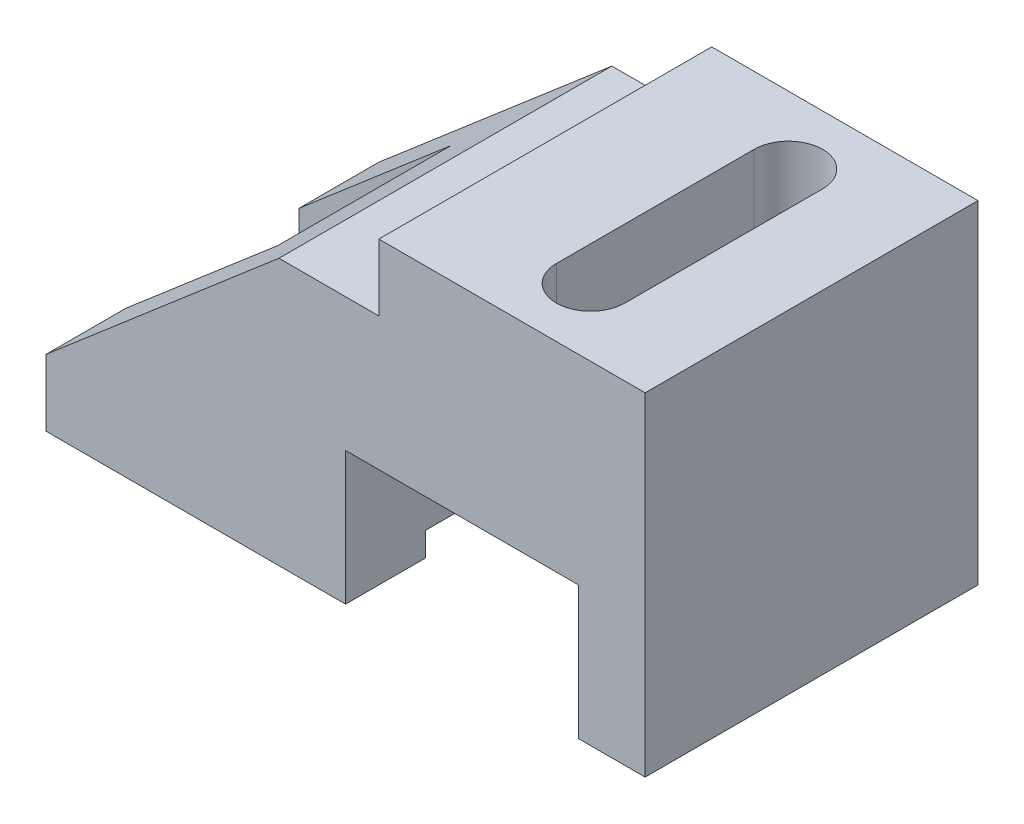
ISO-10303-21;
HEADER;
FILE_DESCRIPTION(('STEP AP214'),'2;1');
FILE_NAME('part.step','',(''),(''),'','','');
FILE_SCHEMA(('AUTOMOTIVE_DESIGN { 1 0 10303 214 1 1 1 1 }'));
ENDSEC;
DATA;
#1=APPLICATION_CONTEXT('core data for automotive mechanical design processes');
#2=APPLICATION_PROTOCOL_DEFINITION('international standard','automotive_design',2000,#1);
#3=PRODUCT_CONTEXT('',#1,'mechanical');
#4=PRODUCT('Part','Part','',(#3));
#5=PRODUCT_RELATED_PRODUCT_CATEGORY('part','',(#4));
#6=PRODUCT_DEFINITION_FORMATION('','',#4);
#7=PRODUCT_DEFINITION_CONTEXT('part definition',#1,'design');
#8=PRODUCT_DEFINITION('design','',#6,#7);
#9=PRODUCT_DEFINITION_SHAPE('','',#8);
#10=(LENGTH_UNIT() NAMED_UNIT(*) SI_UNIT(.MILLI.,.METRE.));
#11=(NAMED_UNIT(*) PLANE_ANGLE_UNIT() SI_UNIT($,.RADIAN.));
#12=(NAMED_UNIT(*) SI_UNIT($,.STERADIAN.) SOLID_ANGLE_UNIT());
#13=UNCERTAINTY_MEASURE_WITH_UNIT(LENGTH_MEASURE(1.E-05),#10,'distance_accuracy_value','');
#14=(GEOMETRIC_REPRESENTATION_CONTEXT(3) GLOBAL_UNCERTAINTY_ASSIGNED_CONTEXT((#13)) GLOBAL_UNIT_ASSIGNED_CONTEXT((#10,
#11,#12)) REPRESENTATION_CONTEXT('',''));
#15=CARTESIAN_POINT('',(0.,0.,0.));
#16=DIRECTION('',(0.,0.,1.));
#17=DIRECTION('',(1.,0.,0.));
#18=AXIS2_PLACEMENT_3D('',#15,#16,#17);
#19=CARTESIAN_POINT('',(0.,0.,50.));
#20=DIRECTION('',(1.,0.,0.));
#21=DIRECTION('',(0.,0.,-1.));
#22=AXIS2_PLACEMENT_3D('',#19,#20,#21);
#23=PLANE('',#22);
#24=DIRECTION('',(0.,0.,-1.));
#25=VECTOR('',#24,1.);
#26=CARTESIAN_POINT('',(0.,10.,50.));
#27=LINE('',#26,#25);
#28=CARTESIAN_POINT('',(0.,10.,50.));
#29=VERTEX_POINT('',#28);
#30=CARTESIAN_POINT('',(0.,10.,38.));
#31=VERTEX_POINT('',#30);
#32=EDGE_CURVE('E198',#29,#31,#27,.T.);
#33=ORIENTED_EDGE('',*,*,#32,.T.);
#34=DIRECTION('',(0.,1.,0.));
#35=VECTOR('',#34,1.);
#36=CARTESIAN_POINT('',(0.,0.,38.));
#37=LINE('',#36,#35);
#38=CARTESIAN_POINT('',(0.,0.,38.));
#39=VERTEX_POINT('',#38);
#40=EDGE_CURVE('E185',#39,#31,#37,.T.);
#41=ORIENTED_EDGE('',*,*,#40,.F.);
#42=DIRECTION('',(0.,0.,-1.));
#43=VECTOR('',#42,1.);
#44=CARTESIAN_POINT('',(0.,0.,50.));
#45=LINE('',#44,#43);
#46=CARTESIAN_POINT('',(0.,0.,50.));
#47=VERTEX_POINT('',#46);
#48=EDGE_CURVE('E11',#47,#39,#45,.T.);
#49=ORIENTED_EDGE('',*,*,#48,.F.);
#50=DIRECTION('',(0.,-1.,0.));
#51=VECTOR('',#50,1.);
#52=CARTESIAN_POINT('',(0.,0.,50.));
#53=LINE('',#52,#51);
#54=EDGE_CURVE('E269',#29,#47,#53,.T.);
#55=ORIENTED_EDGE('',*,*,#54,.F.);
#56=EDGE_LOOP('',(#33,#41,#49,#55));
#57=FACE_BOUND('',#56,.T.);
#58=ADVANCED_FACE('F39',(#57),#23,.F.);
#59=CARTESIAN_POINT('',(0.,0.,50.));
#60=DIRECTION('',(0.,1.,0.));
#61=DIRECTION('',(0.,0.,1.));
#62=AXIS2_PLACEMENT_3D('',#59,#60,#61);
#63=PLANE('',#62);
#64=ORIENTED_EDGE('',*,*,#48,.T.);
#65=DIRECTION('',(1.,0.,0.));
#66=VECTOR('',#65,1.);
#67=CARTESIAN_POINT('',(0.,0.,38.));
#68=LINE('',#67,#66);
#69=CARTESIAN_POINT('',(45.,0.,38.));
#70=VERTEX_POINT('',#69);
#71=EDGE_CURVE('E328',#39,#70,#68,.T.);
#72=ORIENTED_EDGE('',*,*,#71,.T.);
#73=DIRECTION('',(0.,0.,-1.));
#74=VECTOR('',#73,1.);
#75=CARTESIAN_POINT('',(45.,0.,50.));
#76=LINE('',#75,#74);
#77=CARTESIAN_POINT('',(45.,0.,50.));
#78=VERTEX_POINT('',#77);
#79=EDGE_CURVE('E227',#78,#70,#76,.T.);
#80=ORIENTED_EDGE('',*,*,#79,.F.);
#81=DIRECTION('',(1.,0.,0.));
#82=VECTOR('',#81,1.);
#83=CARTESIAN_POINT('',(0.,0.,50.));
#84=LINE('',#83,#82);
#85=EDGE_CURVE('E275',#47,#78,#84,.T.);
#86=ORIENTED_EDGE('',*,*,#85,.F.);
#87=EDGE_LOOP('',(#64,#72,#80,#86));
#88=FACE_BOUND('',#87,.T.);
#89=ADVANCED_FACE('F353',(#88),#63,.F.);
#90=CARTESIAN_POINT('',(0.,0.,12.));
#91=VERTEX_POINT('',#90);
#92=CARTESIAN_POINT('',(0.,0.,0.));
#93=VERTEX_POINT('',#92);
#94=EDGE_CURVE('E50',#91,#93,#45,.T.);
#95=ORIENTED_EDGE('',*,*,#94,.F.);
#96=DIRECTION('',(0.,-1.,0.));
#97=VECTOR('',#96,1.);
#98=CARTESIAN_POINT('',(0.,10.,12.));
#99=LINE('',#98,#97);
#100=CARTESIAN_POINT('',(0.,10.,12.));
#101=VERTEX_POINT('',#100);
#102=EDGE_CURVE('E177',#101,#91,#99,.T.);
#103=ORIENTED_EDGE('',*,*,#102,.F.);
#104=CARTESIAN_POINT('',(0.,10.,0.));
#105=VERTEX_POINT('',#104);
#106=EDGE_CURVE('E178',#101,#105,#27,.T.);
#107=ORIENTED_EDGE('',*,*,#106,.T.);
#108=DIRECTION('',(0.,-1.,0.));
#109=VECTOR('',#108,1.);
#110=CARTESIAN_POINT('',(0.,0.,0.));
#111=LINE('',#110,#109);
#112=EDGE_CURVE('E250',#105,#93,#111,.T.);
#113=ORIENTED_EDGE('',*,*,#112,.T.);
#114=EDGE_LOOP('',(#95,#103,#107,#113));
#115=FACE_BOUND('',#114,.T.);
#116=ADVANCED_FACE('F41',(#115),#23,.F.);
#117=DIRECTION('',(-1.,0.,0.));
#118=VECTOR('',#117,1.);
#119=CARTESIAN_POINT('',(0.,0.,12.));
#120=LINE('',#119,#118);
#121=CARTESIAN_POINT('',(45.,0.,12.));
#122=VERTEX_POINT('',#121);
#123=EDGE_CURVE('E53',#122,#91,#120,.T.);
#124=ORIENTED_EDGE('',*,*,#123,.T.);
#125=ORIENTED_EDGE('',*,*,#94,.T.);
#126=DIRECTION('',(1.,0.,0.));
#127=VECTOR('',#126,1.);
#128=CARTESIAN_POINT('',(0.,0.,0.));
#129=LINE('',#128,#127);
#130=CARTESIAN_POINT('',(45.,0.,0.));
#131=VERTEX_POINT('',#130);
#132=EDGE_CURVE('E245',#93,#131,#129,.T.);
#133=ORIENTED_EDGE('',*,*,#132,.T.);
#134=EDGE_CURVE('E229',#122,#131,#76,.T.);
#135=ORIENTED_EDGE('',*,*,#134,.F.);
#136=EDGE_LOOP('',(#124,#125,#133,#135));
#137=FACE_BOUND('',#136,.T.);
#138=ADVANCED_FACE('F241',(#137),#63,.F.);
#139=CARTESIAN_POINT('',(45.,0.,50.));
#140=DIRECTION('',(-1.,0.,0.));
#141=DIRECTION('',(0.,0.,1.));
#142=AXIS2_PLACEMENT_3D('',#139,#140,#141);
#143=PLANE('',#142);
#144=ORIENTED_EDGE('',*,*,#79,.T.);
#145=DIRECTION('',(0.,1.,0.));
#146=VECTOR('',#145,1.);
#147=CARTESIAN_POINT('',(45.,0.,38.));
#148=LINE('',#147,#146);
#149=CARTESIAN_POINT('',(45.,3.59772228646444,38.));
#150=VERTEX_POINT('',#149);
#151=EDGE_CURVE('E332',#70,#150,#148,.T.);
#152=ORIENTED_EDGE('',*,*,#151,.T.);
#153=DIRECTION('',(0.,0.,-1.));
#154=VECTOR('',#153,1.);
#155=CARTESIAN_POINT('',(45.,3.59772228646444,50.));
#156=LINE('',#155,#154);
#157=CARTESIAN_POINT('',(45.,3.59772228646444,12.));
#158=VERTEX_POINT('',#157);
#159=EDGE_CURVE('E330',#150,#158,#156,.T.);
#160=ORIENTED_EDGE('',*,*,#159,.T.);
#161=DIRECTION('',(0.,-1.,0.));
#162=VECTOR('',#161,1.);
#163=CARTESIAN_POINT('',(45.,0.,12.));
#164=LINE('',#163,#162);
#165=EDGE_CURVE('E243',#158,#122,#164,.T.);
#166=ORIENTED_EDGE('',*,*,#165,.T.);
#167=ORIENTED_EDGE('',*,*,#134,.T.);
#168=DIRECTION('',(0.,1.,0.));
#169=VECTOR('',#168,1.);
#170=CARTESIAN_POINT('',(45.,0.,0.));
#171=LINE('',#170,#169);
#172=CARTESIAN_POINT('',(45.,20.,0.));
#173=VERTEX_POINT('',#172);
#174=EDGE_CURVE('E239',#131,#173,#171,.T.);
#175=ORIENTED_EDGE('',*,*,#174,.T.);
#176=DIRECTION('',(0.,0.,-1.));
#177=VECTOR('',#176,1.);
#178=CARTESIAN_POINT('',(45.,20.,50.));
#179=LINE('',#178,#177);
#180=CARTESIAN_POINT('',(45.,20.,50.));
#181=VERTEX_POINT('',#180);
#182=EDGE_CURVE('E223',#181,#173,#179,.T.);
#183=ORIENTED_EDGE('',*,*,#182,.F.);
#184=DIRECTION('',(0.,1.,0.));
#185=VECTOR('',#184,1.);
#186=CARTESIAN_POINT('',(45.,0.,50.));
#187=LINE('',#186,#185);
#188=EDGE_CURVE('E280',#78,#181,#187,.T.);
#189=ORIENTED_EDGE('',*,*,#188,.F.);
#190=EDGE_LOOP('',(#144,#152,#160,#166,#167,#175,#183,#189));
#191=FACE_BOUND('',#190,.T.);
#192=ADVANCED_FACE('F237',(#191),#143,.F.);
#193=CARTESIAN_POINT('',(45.,20.,50.));
#194=DIRECTION('',(0.,1.,0.));
#195=DIRECTION('',(0.,0.,1.));
#196=AXIS2_PLACEMENT_3D('',#193,#194,#195);
#197=PLANE('',#196);
#198=DIRECTION('',(0.,0.,-1.));
#199=VECTOR('',#198,1.);
#200=CARTESIAN_POINT('',(76.8088026969081,20.,50.));
#201=LINE('',#200,#199);
#202=CARTESIAN_POINT('',(76.8088026969081,20.,39.8529445474259));
#203=VERTEX_POINT('',#202);
#204=CARTESIAN_POINT('',(76.8088026969081,20.,10.1470554525741));
#205=VERTEX_POINT('',#204);
#206=EDGE_CURVE('E299',#203,#205,#201,.T.);
#207=ORIENTED_EDGE('',*,*,#206,.T.);
#208=CARTESIAN_POINT('',(71.6617472443339,20.,10.1470554525741));
#209=DIRECTION('',(0.,1.,0.));
#210=DIRECTION('',(0.,0.,1.));
#211=AXIS2_PLACEMENT_3D('',#208,#209,#210);
#212=CIRCLE('',#211,5.14705545257413);
#213=CARTESIAN_POINT('',(66.5146917917598,20.,10.1470554525741));
#214=VERTEX_POINT('',#213);
#215=EDGE_CURVE('E278',#205,#214,#212,.T.);
#216=ORIENTED_EDGE('',*,*,#215,.T.);
#217=DIRECTION('',(0.,0.,1.));
#218=VECTOR('',#217,1.);
#219=CARTESIAN_POINT('',(66.5146917917598,20.,50.));
#220=LINE('',#219,#218);
#221=CARTESIAN_POINT('',(66.5146917917598,20.,39.8529445474259));
#222=VERTEX_POINT('',#221);
#223=EDGE_CURVE('E304',#214,#222,#220,.T.);
#224=ORIENTED_EDGE('',*,*,#223,.T.);
#225=CARTESIAN_POINT('',(71.6617472443339,20.,39.8529445474259));
#226=DIRECTION('',(0.,1.,0.));
#227=DIRECTION('',(0.,0.,1.));
#228=AXIS2_PLACEMENT_3D('',#225,#226,#227);
#229=CIRCLE('',#228,5.14705545257414);
#230=EDGE_CURVE('E302',#222,#203,#229,.T.);
#231=ORIENTED_EDGE('',*,*,#230,.T.);
#232=EDGE_LOOP('',(#207,#216,#224,#231));
#233=FACE_BOUND('',#232,.T.);
#234=DIRECTION('',(1.,0.,0.));
#235=VECTOR('',#234,1.);
#236=CARTESIAN_POINT('',(45.,20.,0.));
#237=LINE('',#236,#235);
#238=CARTESIAN_POINT('',(80.,20.,0.));
#239=VERTEX_POINT('',#238);
#240=EDGE_CURVE('E252',#173,#239,#237,.T.);
#241=ORIENTED_EDGE('',*,*,#240,.T.);
#242=DIRECTION('',(0.,0.,-1.));
#243=VECTOR('',#242,1.);
#244=CARTESIAN_POINT('',(80.,20.,50.));
#245=LINE('',#244,#243);
#246=CARTESIAN_POINT('',(80.,20.,50.));
#247=VERTEX_POINT('',#246);
#248=EDGE_CURVE('E225',#247,#239,#245,.T.);
#249=ORIENTED_EDGE('',*,*,#248,.F.);
#250=DIRECTION('',(1.,0.,0.));
#251=VECTOR('',#250,1.);
#252=CARTESIAN_POINT('',(45.,20.,50.));
#253=LINE('',#252,#251);
#254=EDGE_CURVE('E285',#181,#247,#253,.T.);
#255=ORIENTED_EDGE('',*,*,#254,.F.);
#256=ORIENTED_EDGE('',*,*,#182,.T.);
#257=EDGE_LOOP('',(#241,#249,#255,#256));
#258=FACE_BOUND('',#257,.T.);
#259=ADVANCED_FACE('F357',(#233,#258),#197,.F.);
#260=CARTESIAN_POINT('',(80.,20.,50.));
#261=DIRECTION('',(1.,0.,0.));
#262=DIRECTION('',(0.,0.,-1.));
#263=AXIS2_PLACEMENT_3D('',#260,#261,#262);
#264=PLANE('',#263);
#265=DIRECTION('',(0.,-1.,0.));
#266=VECTOR('',#265,1.);
#267=CARTESIAN_POINT('',(80.,20.,0.));
#268=LINE('',#267,#266);
#269=CARTESIAN_POINT('',(80.,0.,0.));
#270=VERTEX_POINT('',#269);
#271=EDGE_CURVE('E255',#239,#270,#268,.T.);
#272=ORIENTED_EDGE('',*,*,#271,.T.);
#273=DIRECTION('',(0.,0.,-1.));
#274=VECTOR('',#273,1.);
#275=CARTESIAN_POINT('',(80.,0.,50.));
#276=LINE('',#275,#274);
#277=CARTESIAN_POINT('',(80.,0.,50.));
#278=VERTEX_POINT('',#277);
#279=EDGE_CURVE('E218',#278,#270,#276,.T.);
#280=ORIENTED_EDGE('',*,*,#279,.F.);
#281=DIRECTION('',(0.,-1.,0.));
#282=VECTOR('',#281,1.);
#283=CARTESIAN_POINT('',(80.,20.,50.));
#284=LINE('',#283,#282);
#285=EDGE_CURVE('E287',#247,#278,#284,.T.);
#286=ORIENTED_EDGE('',*,*,#285,.F.);
#287=ORIENTED_EDGE('',*,*,#248,.T.);
#288=EDGE_LOOP('',(#272,#280,#286,#287));
#289=FACE_BOUND('',#288,.T.);
#290=ADVANCED_FACE('F358',(#289),#264,.F.);
#291=CARTESIAN_POINT('',(80.,0.,50.));
#292=DIRECTION('',(0.,1.,0.));
#293=DIRECTION('',(0.,0.,1.));
#294=AXIS2_PLACEMENT_3D('',#291,#292,#293);
#295=PLANE('',#294);
#296=DIRECTION('',(1.,0.,0.));
#297=VECTOR('',#296,1.);
#298=CARTESIAN_POINT('',(80.,0.,0.));
#299=LINE('',#298,#297);
#300=CARTESIAN_POINT('',(90.,0.,0.));
#301=VERTEX_POINT('',#300);
#302=EDGE_CURVE('E259',#270,#301,#299,.T.);
#303=ORIENTED_EDGE('',*,*,#302,.T.);
#304=DIRECTION('',(0.,0.,-1.));
#305=VECTOR('',#304,1.);
#306=CARTESIAN_POINT('',(90.,0.,50.));
#307=LINE('',#306,#305);
#308=CARTESIAN_POINT('',(90.,0.,50.));
#309=VERTEX_POINT('',#308);
#310=EDGE_CURVE('E216',#309,#301,#307,.T.);
#311=ORIENTED_EDGE('',*,*,#310,.F.);
#312=DIRECTION('',(1.,0.,0.));
#313=VECTOR('',#312,1.);
#314=CARTESIAN_POINT('',(80.,0.,50.));
#315=LINE('',#314,#313);
#316=EDGE_CURVE('E289',#278,#309,#315,.T.);
#317=ORIENTED_EDGE('',*,*,#316,.F.);
#318=ORIENTED_EDGE('',*,*,#279,.T.);
#319=EDGE_LOOP('',(#303,#311,#317,#318));
#320=FACE_BOUND('',#319,.T.);
#321=ADVANCED_FACE('F368',(#320),#295,.F.);
#322=CARTESIAN_POINT('',(90.,0.,50.));
#323=DIRECTION('',(-1.,0.,0.));
#324=DIRECTION('',(0.,0.,1.));
#325=AXIS2_PLACEMENT_3D('',#322,#323,#324);
#326=PLANE('',#325);
#327=DIRECTION('',(0.,1.,0.));
#328=VECTOR('',#327,1.);
#329=CARTESIAN_POINT('',(90.,0.,0.));
#330=LINE('',#329,#328);
#331=CARTESIAN_POINT('',(90.,50.,0.));
#332=VERTEX_POINT('',#331);
#333=EDGE_CURVE('E261',#301,#332,#330,.T.);
#334=ORIENTED_EDGE('',*,*,#333,.T.);
#335=DIRECTION('',(0.,0.,-1.));
#336=VECTOR('',#335,1.);
#337=CARTESIAN_POINT('',(90.,50.,50.));
#338=LINE('',#337,#336);
#339=CARTESIAN_POINT('',(90.,50.,50.));
#340=VERTEX_POINT('',#339);
#341=EDGE_CURVE('E213',#340,#332,#338,.T.);
#342=ORIENTED_EDGE('',*,*,#341,.F.);
#343=DIRECTION('',(0.,1.,0.));
#344=VECTOR('',#343,1.);
#345=CARTESIAN_POINT('',(90.,0.,50.));
#346=LINE('',#345,#344);
#347=EDGE_CURVE('E288',#309,#340,#346,.T.);
#348=ORIENTED_EDGE('',*,*,#347,.F.);
#349=ORIENTED_EDGE('',*,*,#310,.T.);
#350=EDGE_LOOP('',(#334,#342,#348,#349));
#351=FACE_BOUND('',#350,.T.);
#352=ADVANCED_FACE('F367',(#351),#326,.F.);
#353=CARTESIAN_POINT('',(90.,50.,50.));
#354=DIRECTION('',(0.,-1.,0.));
#355=DIRECTION('',(0.,0.,-1.));
#356=AXIS2_PLACEMENT_3D('',#353,#354,#355);
#357=PLANE('',#356);
#358=DIRECTION('',(0.,0.,1.));
#359=VECTOR('',#358,1.);
#360=CARTESIAN_POINT('',(66.5146917917598,50.,10.1470554525741));
#361=LINE('',#360,#359);
#362=CARTESIAN_POINT('',(66.5146917917598,50.,10.1470554525741));
#363=VERTEX_POINT('',#362);
#364=CARTESIAN_POINT('',(66.5146917917598,50.,39.8529445474259));
#365=VERTEX_POINT('',#364);
#366=EDGE_CURVE('E325',#363,#365,#361,.T.);
#367=ORIENTED_EDGE('',*,*,#366,.F.);
#368=CARTESIAN_POINT('',(71.6617472443339,50.,10.1470554525741));
#369=DIRECTION('',(0.,1.,0.));
#370=DIRECTION('',(0.,0.,1.));
#371=AXIS2_PLACEMENT_3D('',#368,#369,#370);
#372=CIRCLE('',#371,5.14705545257413);
#373=CARTESIAN_POINT('',(76.8088026969081,50.,10.1470554525741));
#374=VERTEX_POINT('',#373);
#375=EDGE_CURVE('E324',#374,#363,#372,.T.);
#376=ORIENTED_EDGE('',*,*,#375,.F.);
#377=DIRECTION('',(0.,0.,-1.));
#378=VECTOR('',#377,1.);
#379=CARTESIAN_POINT('',(76.8088026969081,50.,10.1470554525741));
#380=LINE('',#379,#378);
#381=CARTESIAN_POINT('',(76.8088026969081,50.,39.8529445474259));
#382=VERTEX_POINT('',#381);
#383=EDGE_CURVE('E315',#382,#374,#380,.T.);
#384=ORIENTED_EDGE('',*,*,#383,.F.);
#385=CARTESIAN_POINT('',(71.6617472443339,50.,39.8529445474259));
#386=DIRECTION('',(0.,1.,0.));
#387=DIRECTION('',(0.,0.,1.));
#388=AXIS2_PLACEMENT_3D('',#385,#386,#387);
#389=CIRCLE('',#388,5.14705545257414);
#390=EDGE_CURVE('E317',#365,#382,#389,.T.);
#391=ORIENTED_EDGE('',*,*,#390,.F.);
#392=EDGE_LOOP('',(#367,#376,#384,#391));
#393=FACE_BOUND('',#392,.T.);
#394=DIRECTION('',(-1.,0.,0.));
#395=VECTOR('',#394,1.);
#396=CARTESIAN_POINT('',(90.,50.,0.));
#397=LINE('',#396,#395);
#398=CARTESIAN_POINT('',(50.,50.,0.));
#399=VERTEX_POINT('',#398);
#400=EDGE_CURVE('E263',#332,#399,#397,.T.);
#401=ORIENTED_EDGE('',*,*,#400,.T.);
#402=DIRECTION('',(0.,0.,-1.));
#403=VECTOR('',#402,1.);
#404=CARTESIAN_POINT('',(50.,50.,50.));
#405=LINE('',#404,#403);
#406=CARTESIAN_POINT('',(50.,50.,50.));
#407=VERTEX_POINT('',#406);
#408=EDGE_CURVE('E209',#407,#399,#405,.T.);
#409=ORIENTED_EDGE('',*,*,#408,.F.);
#410=DIRECTION('',(-1.,0.,0.));
#411=VECTOR('',#410,1.);
#412=CARTESIAN_POINT('',(90.,50.,50.));
#413=LINE('',#412,#411);
#414=EDGE_CURVE('E295',#340,#407,#413,.T.);
#415=ORIENTED_EDGE('',*,*,#414,.F.);
#416=ORIENTED_EDGE('',*,*,#341,.T.);
#417=EDGE_LOOP('',(#401,#409,#415,#416));
#418=FACE_BOUND('',#417,.T.);
#419=ADVANCED_FACE('F374',(#393,#418),#357,.F.);
#420=CARTESIAN_POINT('',(50.,50.,50.));
#421=DIRECTION('',(1.,0.,0.));
#422=DIRECTION('',(0.,0.,-1.));
#423=AXIS2_PLACEMENT_3D('',#420,#421,#422);
#424=PLANE('',#423);
#425=DIRECTION('',(0.,-1.,0.));
#426=VECTOR('',#425,1.);
#427=CARTESIAN_POINT('',(50.,50.,0.));
#428=LINE('',#427,#426);
#429=CARTESIAN_POINT('',(50.,40.,0.));
#430=VERTEX_POINT('',#429);
#431=EDGE_CURVE('E264',#399,#430,#428,.T.);
#432=ORIENTED_EDGE('',*,*,#431,.T.);
#433=DIRECTION('',(0.,0.,-1.));
#434=VECTOR('',#433,1.);
#435=CARTESIAN_POINT('',(50.,40.,50.));
#436=LINE('',#435,#434);
#437=CARTESIAN_POINT('',(50.,40.,50.));
#438=VERTEX_POINT('',#437);
#439=EDGE_CURVE('E210',#438,#430,#436,.T.);
#440=ORIENTED_EDGE('',*,*,#439,.F.);
#441=DIRECTION('',(0.,-1.,0.));
#442=VECTOR('',#441,1.);
#443=CARTESIAN_POINT('',(50.,50.,50.));
#444=LINE('',#443,#442);
#445=EDGE_CURVE('E294',#407,#438,#444,.T.);
#446=ORIENTED_EDGE('',*,*,#445,.F.);
#447=ORIENTED_EDGE('',*,*,#408,.T.);
#448=EDGE_LOOP('',(#432,#440,#446,#447));
#449=FACE_BOUND('',#448,.T.);
#450=ADVANCED_FACE('F379',(#449),#424,.F.);
#451=CARTESIAN_POINT('',(50.,40.,50.));
#452=DIRECTION('',(0.,-1.,0.));
#453=DIRECTION('',(0.,0.,-1.));
#454=AXIS2_PLACEMENT_3D('',#451,#452,#453);
#455=PLANE('',#454);
#456=DIRECTION('',(-1.,0.,0.));
#457=VECTOR('',#456,1.);
#458=CARTESIAN_POINT('',(50.,40.,0.));
#459=LINE('',#458,#457);
#460=CARTESIAN_POINT('',(35.,40.,0.));
#461=VERTEX_POINT('',#460);
#462=EDGE_CURVE('E266',#430,#461,#459,.T.);
#463=ORIENTED_EDGE('',*,*,#462,.T.);
#464=DIRECTION('',(0.,0.,-1.));
#465=VECTOR('',#464,1.);
#466=CARTESIAN_POINT('',(35.,40.,50.));
#467=LINE('',#466,#465);
#468=CARTESIAN_POINT('',(35.,40.,50.));
#469=VERTEX_POINT('',#468);
#470=EDGE_CURVE('E199',#469,#461,#467,.T.);
#471=ORIENTED_EDGE('',*,*,#470,.F.);
#472=DIRECTION('',(-1.,0.,0.));
#473=VECTOR('',#472,1.);
#474=CARTESIAN_POINT('',(50.,40.,50.));
#475=LINE('',#474,#473);
#476=EDGE_CURVE('E203',#438,#469,#475,.T.);
#477=ORIENTED_EDGE('',*,*,#476,.F.);
#478=ORIENTED_EDGE('',*,*,#439,.T.);
#479=EDGE_LOOP('',(#463,#471,#477,#478));
#480=FACE_BOUND('',#479,.T.);
#481=ADVANCED_FACE('F385',(#480),#455,.F.);
#482=CARTESIAN_POINT('',(0.,10.,50.));
#483=DIRECTION('',(0.650791373455968,-0.759256602365297,0.));
#484=DIRECTION('',(0.759256602365297,0.650791373455968,0.));
#485=AXIS2_PLACEMENT_3D('',#482,#483,#484);
#486=PLANE('',#485);
#487=DIRECTION('',(0.,0.,-1.));
#488=VECTOR('',#487,1.);
#489=CARTESIAN_POINT('',(22.7776980709589,29.5237412036791,12.));
#490=LINE('',#489,#488);
#491=CARTESIAN_POINT('',(22.7776980709589,29.5237412036791,38.));
#492=VERTEX_POINT('',#491);
#493=CARTESIAN_POINT('',(22.7776980709589,29.5237412036791,12.));
#494=VERTEX_POINT('',#493);
#495=EDGE_CURVE('E64',#492,#494,#490,.T.);
#496=ORIENTED_EDGE('',*,*,#495,.F.);
#497=DIRECTION('',(0.759256602365297,0.650791373455968,0.));
#498=VECTOR('',#497,1.);
#499=CARTESIAN_POINT('',(0.,10.,38.));
#500=LINE('',#499,#498);
#501=EDGE_CURVE('E190',#31,#492,#500,.T.);
#502=ORIENTED_EDGE('',*,*,#501,.F.);
#503=ORIENTED_EDGE('',*,*,#32,.F.);
#504=DIRECTION('',(-0.759256602365297,-0.650791373455968,0.));
#505=VECTOR('',#504,1.);
#506=CARTESIAN_POINT('',(0.,10.,50.));
#507=LINE('',#506,#505);
#508=EDGE_CURVE('E197',#469,#29,#507,.T.);
#509=ORIENTED_EDGE('',*,*,#508,.F.);
#510=ORIENTED_EDGE('',*,*,#470,.T.);
#511=DIRECTION('',(-0.759256602365297,-0.650791373455968,0.));
#512=VECTOR('',#511,1.);
#513=CARTESIAN_POINT('',(0.,10.,0.));
#514=LINE('',#513,#512);
#515=EDGE_CURVE('E191',#461,#105,#514,.T.);
#516=ORIENTED_EDGE('',*,*,#515,.T.);
#517=ORIENTED_EDGE('',*,*,#106,.F.);
#518=DIRECTION('',(-0.759256602365297,-0.650791373455969,0.));
#519=VECTOR('',#518,1.);
#520=CARTESIAN_POINT('',(0.,10.,12.));
#521=LINE('',#520,#519);
#522=EDGE_CURVE('E183',#494,#101,#521,.T.);
#523=ORIENTED_EDGE('',*,*,#522,.F.);
#524=EDGE_LOOP('',(#496,#502,#503,#509,#510,#516,#517,#523));
#525=FACE_BOUND('',#524,.T.);
#526=ADVANCED_FACE('F192',(#525),#486,.F.);
#527=CARTESIAN_POINT('',(0.,0.,50.));
#528=DIRECTION('',(0.,0.,1.));
#529=DIRECTION('',(1.,0.,0.));
#530=AXIS2_PLACEMENT_3D('',#527,#528,#529);
#531=PLANE('',#530);
#532=ORIENTED_EDGE('',*,*,#54,.T.);
#533=ORIENTED_EDGE('',*,*,#85,.T.);
#534=ORIENTED_EDGE('',*,*,#188,.T.);
#535=ORIENTED_EDGE('',*,*,#254,.T.);
#536=ORIENTED_EDGE('',*,*,#285,.T.);
#537=ORIENTED_EDGE('',*,*,#316,.T.);
#538=ORIENTED_EDGE('',*,*,#347,.T.);
#539=ORIENTED_EDGE('',*,*,#414,.T.);
#540=ORIENTED_EDGE('',*,*,#445,.T.);
#541=ORIENTED_EDGE('',*,*,#476,.T.);
#542=ORIENTED_EDGE('',*,*,#508,.T.);
#543=EDGE_LOOP('',(#532,#533,#534,#535,#536,#537,#538,#539,#540,#541,#542));
#544=FACE_BOUND('',#543,.T.);
#545=ADVANCED_FACE('F354',(#544),#531,.T.);
#546=CARTESIAN_POINT('',(0.,0.,0.));
#547=DIRECTION('',(0.,0.,1.));
#548=DIRECTION('',(1.,0.,0.));
#549=AXIS2_PLACEMENT_3D('',#546,#547,#548);
#550=PLANE('',#549);
#551=ORIENTED_EDGE('',*,*,#112,.F.);
#552=ORIENTED_EDGE('',*,*,#515,.F.);
#553=ORIENTED_EDGE('',*,*,#462,.F.);
#554=ORIENTED_EDGE('',*,*,#431,.F.);
#555=ORIENTED_EDGE('',*,*,#400,.F.);
#556=ORIENTED_EDGE('',*,*,#333,.F.);
#557=ORIENTED_EDGE('',*,*,#302,.F.);
#558=ORIENTED_EDGE('',*,*,#271,.F.);
#559=ORIENTED_EDGE('',*,*,#240,.F.);
#560=ORIENTED_EDGE('',*,*,#174,.F.);
#561=ORIENTED_EDGE('',*,*,#132,.F.);
#562=EDGE_LOOP('',(#551,#552,#553,#554,#555,#556,#557,#558,#559,#560,#561));
#563=FACE_BOUND('',#562,.T.);
#564=ADVANCED_FACE('F248',(#563),#550,.F.);
#565=CARTESIAN_POINT('',(71.6617472443339,16.,10.1470554525741));
#566=DIRECTION('',(0.,1.,0.));
#567=DIRECTION('',(0.,0.,1.));
#568=AXIS2_PLACEMENT_3D('',#565,#566,#567);
#569=CYLINDRICAL_SURFACE('',#568,5.14705545257413);
#570=DIRECTION('',(0.,1.,0.));
#571=VECTOR('',#570,1.);
#572=CARTESIAN_POINT('',(76.8088026969081,16.,10.1470554525741));
#573=LINE('',#572,#571);
#574=EDGE_CURVE('E307',#205,#374,#573,.T.);
#575=ORIENTED_EDGE('',*,*,#574,.T.);
#576=ORIENTED_EDGE('',*,*,#375,.T.);
#577=DIRECTION('',(0.,1.,0.));
#578=VECTOR('',#577,1.);
#579=CARTESIAN_POINT('',(66.5146917917598,16.,10.1470554525741));
#580=LINE('',#579,#578);
#581=EDGE_CURVE('E306',#214,#363,#580,.T.);
#582=ORIENTED_EDGE('',*,*,#581,.F.);
#583=ORIENTED_EDGE('',*,*,#215,.F.);
#584=EDGE_LOOP('',(#575,#576,#582,#583));
#585=FACE_BOUND('',#584,.T.);
#586=ADVANCED_FACE('F428',(#585),#569,.F.);
#587=CARTESIAN_POINT('',(76.8088026969081,16.,10.1470554525741));
#588=DIRECTION('',(1.,0.,0.));
#589=DIRECTION('',(0.,0.,-1.));
#590=AXIS2_PLACEMENT_3D('',#587,#588,#589);
#591=PLANE('',#590);
#592=DIRECTION('',(0.,1.,0.));
#593=VECTOR('',#592,1.);
#594=CARTESIAN_POINT('',(76.8088026969081,16.,39.8529445474259));
#595=LINE('',#594,#593);
#596=EDGE_CURVE('E314',#203,#382,#595,.T.);
#597=ORIENTED_EDGE('',*,*,#596,.T.);
#598=ORIENTED_EDGE('',*,*,#383,.T.);
#599=ORIENTED_EDGE('',*,*,#574,.F.);
#600=ORIENTED_EDGE('',*,*,#206,.F.);
#601=EDGE_LOOP('',(#597,#598,#599,#600));
#602=FACE_BOUND('',#601,.T.);
#603=ADVANCED_FACE('F431',(#602),#591,.F.);
#604=CARTESIAN_POINT('',(71.6617472443339,16.,39.8529445474259));
#605=DIRECTION('',(0.,1.,0.));
#606=DIRECTION('',(0.,0.,1.));
#607=AXIS2_PLACEMENT_3D('',#604,#605,#606);
#608=CYLINDRICAL_SURFACE('',#607,5.14705545257414);
#609=DIRECTION('',(0.,1.,0.));
#610=VECTOR('',#609,1.);
#611=CARTESIAN_POINT('',(66.5146917917598,16.,39.8529445474259));
#612=LINE('',#611,#610);
#613=EDGE_CURVE('E313',#222,#365,#612,.T.);
#614=ORIENTED_EDGE('',*,*,#613,.T.);
#615=ORIENTED_EDGE('',*,*,#390,.T.);
#616=ORIENTED_EDGE('',*,*,#596,.F.);
#617=ORIENTED_EDGE('',*,*,#230,.F.);
#618=EDGE_LOOP('',(#614,#615,#616,#617));
#619=FACE_BOUND('',#618,.T.);
#620=ADVANCED_FACE('F432',(#619),#608,.F.);
#621=CARTESIAN_POINT('',(66.5146917917598,16.,10.1470554525741));
#622=DIRECTION('',(-1.,0.,0.));
#623=DIRECTION('',(0.,0.,1.));
#624=AXIS2_PLACEMENT_3D('',#621,#622,#623);
#625=PLANE('',#624);
#626=ORIENTED_EDGE('',*,*,#581,.T.);
#627=ORIENTED_EDGE('',*,*,#366,.T.);
#628=ORIENTED_EDGE('',*,*,#613,.F.);
#629=ORIENTED_EDGE('',*,*,#223,.F.);
#630=EDGE_LOOP('',(#626,#627,#628,#629));
#631=FACE_BOUND('',#630,.T.);
#632=ADVANCED_FACE('F424',(#631),#625,.F.);
#633=CARTESIAN_POINT('',(65.8365216003707,-20.711552913968,12.));
#634=DIRECTION('',(0.759256602365297,0.650791373455969,0.));
#635=DIRECTION('',(-0.650791373455969,0.759256602365297,0.));
#636=AXIS2_PLACEMENT_3D('',#633,#634,#635);
#637=PLANE('',#636);
#638=DIRECTION('',(-0.650791373455969,0.759256602365297,0.));
#639=VECTOR('',#638,1.);
#640=CARTESIAN_POINT('',(65.8365216003707,-20.711552913968,38.));
#641=LINE('',#640,#639);
#642=EDGE_CURVE('E333',#150,#492,#641,.T.);
#643=ORIENTED_EDGE('',*,*,#642,.T.);
#644=ORIENTED_EDGE('',*,*,#495,.T.);
#645=DIRECTION('',(-0.650791373455969,0.759256602365297,0.));
#646=VECTOR('',#645,1.);
#647=CARTESIAN_POINT('',(65.8365216003707,-20.711552913968,12.));
#648=LINE('',#647,#646);
#649=EDGE_CURVE('E189',#158,#494,#648,.T.);
#650=ORIENTED_EDGE('',*,*,#649,.F.);
#651=ORIENTED_EDGE('',*,*,#159,.F.);
#652=EDGE_LOOP('',(#643,#644,#650,#651));
#653=FACE_BOUND('',#652,.T.);
#654=ADVANCED_FACE('F442',(#653),#637,.F.);
#655=CARTESIAN_POINT('',(43.0588235294118,-40.2352941176471,38.));
#656=DIRECTION('',(0.,0.,1.));
#657=DIRECTION('',(1.,0.,0.));
#658=AXIS2_PLACEMENT_3D('',#655,#656,#657);
#659=PLANE('',#658);
#660=ORIENTED_EDGE('',*,*,#40,.T.);
#661=ORIENTED_EDGE('',*,*,#501,.T.);
#662=ORIENTED_EDGE('',*,*,#642,.F.);
#663=ORIENTED_EDGE('',*,*,#151,.F.);
#664=ORIENTED_EDGE('',*,*,#71,.F.);
#665=EDGE_LOOP('',(#660,#661,#662,#663,#664));
#666=FACE_BOUND('',#665,.T.);
#667=ADVANCED_FACE('F341',(#666),#659,.F.);
#668=CARTESIAN_POINT('',(43.0588235294118,-40.2352941176471,12.));
#669=DIRECTION('',(0.,0.,-1.));
#670=DIRECTION('',(-1.,0.,0.));
#671=AXIS2_PLACEMENT_3D('',#668,#669,#670);
#672=PLANE('',#671);
#673=ORIENTED_EDGE('',*,*,#522,.T.);
#674=ORIENTED_EDGE('',*,*,#102,.T.);
#675=ORIENTED_EDGE('',*,*,#123,.F.);
#676=ORIENTED_EDGE('',*,*,#165,.F.);
#677=ORIENTED_EDGE('',*,*,#649,.T.);
#678=EDGE_LOOP('',(#673,#674,#675,#676,#677));
#679=FACE_BOUND('',#678,.T.);
#680=ADVANCED_FACE('F188',(#679),#672,.F.);
#681=CLOSED_SHELL('',(#58,#89,#116,#138,#192,#259,#290,#321,#352,#419,#450,#481,#526,#545,#564,
#586,#603,#620,#632,#654,#667,#680));
#682=MANIFOLD_SOLID_BREP('B2',#681);
#683=ADVANCED_BREP_SHAPE_REPRESENTATION('',(#18,#682),#14);
#684=SHAPE_DEFINITION_REPRESENTATION(#9,#683);
ENDSEC;
END-ISO-10303-21;
